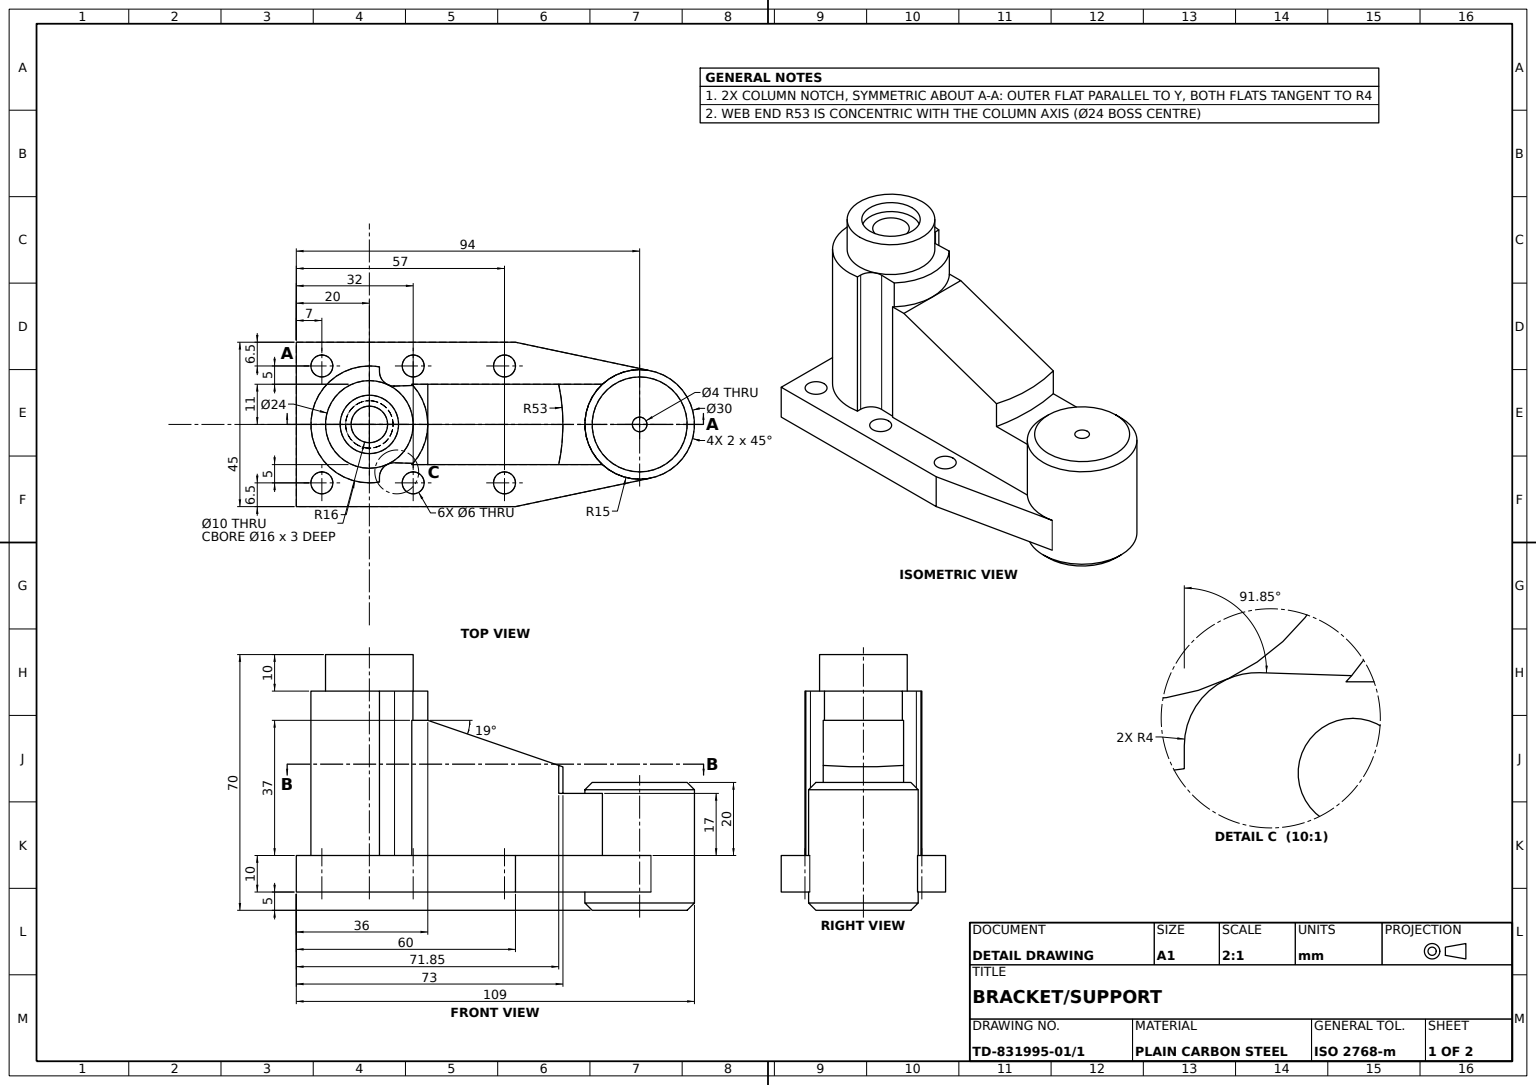
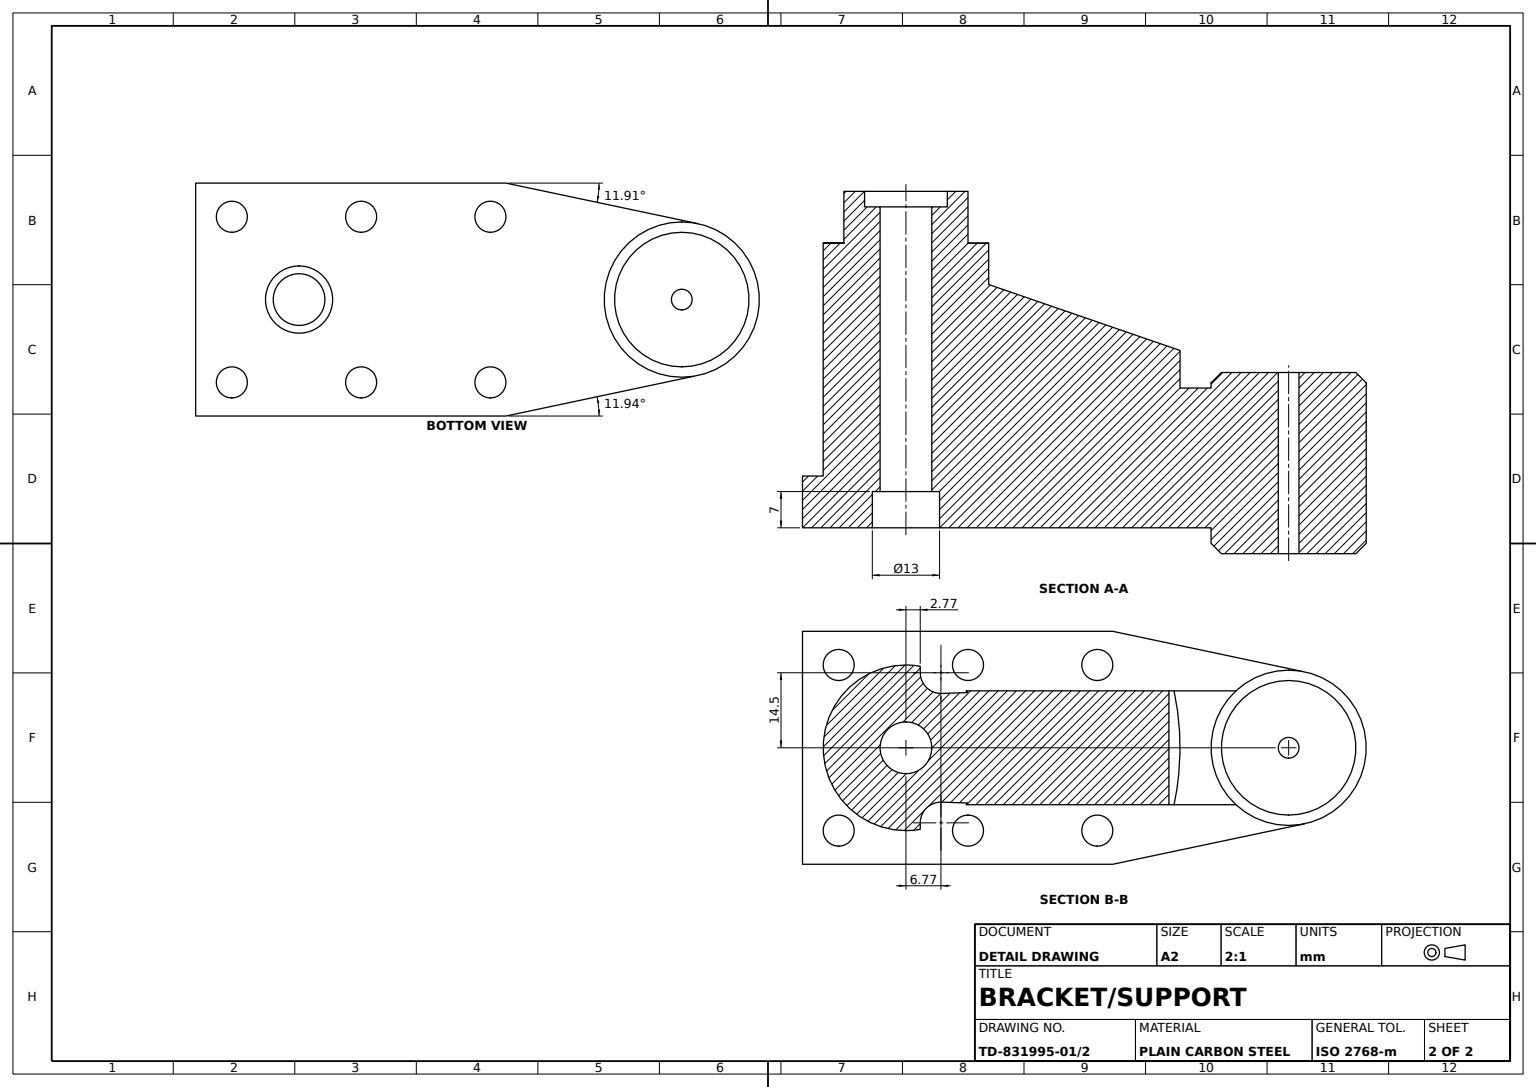
SolidWorks part; units mm, degrees
material "Plain Carbon Steel"
ref_plane "Front Plane" through (0, 0, 0) normal (0, 0, 1) x (1, 0, 0)
ref_plane "Top Plane" through (0, 0, 0) normal (0, 1, 0) x (1, 0, 0)
ref_plane "Right Plane" through (0, 0, 0) normal (1, 0, 0) x (0, 0, -1)
sketch "Pivot Hub Sketch" plane through (0, 0, 0) normal (0, 1, 0) x (1, 0, 0)
  circle A0 centre (0, 0) radius 15
  dimension "D1" = 30
extrude "Pivot Hub Ø30" add sketch "Pivot Hub Sketch" along normal blind 35
ref_plane "Plane1" through (0, 5, 0) normal (0, 1, 0) x (1, 0, 0)
sketch "Base Plate Sketch" plane through (0, 5, 0) normal (0, 1, 0) x (1, 0, 0)
  line L1 (-94, 0) -> (-94, 22.5)
  line L2 (-94, 22.5) -> (-34, 22.5)
  line L3 (-34, 22.5) -> (2.3279, 14.8183)
  line L4 (-94, 0) -> (-94, -22.5)
  line L5 (-94, -22.5) -> (-34, -22.5)
  line L6 (-34, -22.5) -> (3.0952, -14.6772)
  circle A0 centre (0, 0) radius 15 construction
  arc A1 (2.3279, 14.8183) -> (3.0952, -14.6772) centre (0, 0) ccw
  dimension "D1" = 45
  dimension "D2" = 60
  dimension "D3" = 36.3279
  dimension "D4" = 94
  dimension "D5" = 22.5
  dimension "D6" = 40.7707
  dimension "D7" = 94
  dimension "D8" = 37.0952
extrude "Base Plate" add sketch "Base Plate Sketch" along normal blind 10
sketch "Column Sketch" plane through (0, 15, 0) normal (0, 1, 0) x (1, 0, 0)
  circle A0 centre (-74, 0) radius 16
  dimension "D1" = 32
  dimension "D2" = 74
extrude "Column Ø32" add sketch "Column Sketch" along normal blind 45
sketch "Web Sketch" plane through (0, 15, 0) normal (0, 1, 0) x (1, 0, 0)
  line L0 (-74, 11) -> (-22.1541, 11)
  line L1 (-74, -11) -> (-22.1541, -11)
  arc A0 (-74, 11) -> (-74, -11) centre (-74, 0) ccw
  arc A1 (-22.1541, -11) -> (-22.1541, 11) centre (-74, 0) ccw
  dimension "D1" = 11
  dimension "D2" = 53
extrude "Sloped Web" add sketch "Web Sketch" along normal blind 37
sketch "Web Trim Sketch" plane through (0, 0, 11) normal (0, 0, 1) x (1, 0, 0)
  line L2 (-62.381, 52) -> (-62.381, 15) construction
  line L3 (-58, 52) -> (-22.1541, 52)
  line L7 (-58, 52) -> (-16.5018, 37.711)
  line L8 (-22.1541, 52) -> (-16.5018, 52)
  line L9 (-16.5018, 52) -> (-16.5018, 37.711)
  line L10 (-62.381, 52) -> (-22.1541, 52) construction
  dimension "D1" = 45.8793
  dimension "D2" = 14.289
extrude "Web Trim Cut" cut sketch "Web Trim Sketch" against normal blind 37
sketch "Web Pad Sketch" plane through (0, 15, 0) normal (0, 1, 0) x (1, 0, 0)
  line L0 (-22.1541, 11) -> (-1.8695, 11)
  line L1 (-1.8695, 11) -> (-1.8695, -11)
  line L2 (-1.8695, -11) -> (-22.1541, -11)
  arc A0 (-22.1541, 11) -> (-22.1541, -11) centre (-74, 0) cw
  dimension "D1" = 53
  dimension "D2" = 72.1305
extrude "Web Pad" add sketch "Web Pad Sketch" along normal blind 17
chamfer "Hub Chamfer A" distance 2 angle 45 1 edges at (0, 35, 15)
chamfer "Hub Chamfer B" distance 2 angle 45 1 edges at (0, 0, 15)
sketch "Hub Pin Hole Sketch" plane through (0, 35, 0) normal (0, 1, 0) x (1, 0, 0)
  circle A0 centre (0, 0) radius 2
  dimension "D1" = 4
extrude "Hub Pin Hole Ø4" cut sketch "Hub Pin Hole Sketch" against normal blind 39
sketch "Column Top Boss Sketch" plane through (0, 60, 0) normal (0, 1, 0) x (1, 0, 0)
  circle A0 centre (-74, 0) radius 12
  dimension "D1" = 24
extrude "Column Top Boss Ø24" add sketch "Column Top Boss Sketch" along normal blind 10
sketch "Top Counterbore Sketch" plane through (0, 70, 0) normal (0, 1, 0) x (1, 0, 0)
  circle A0 centre (-74, 0) radius 8
  dimension "D1" = 16
extrude "Top Counterbore Ø16" cut sketch "Top Counterbore Sketch" against normal blind 3
sketch "Column Bore Sketch" plane through (0, 67, 0) normal (0, 1, 0) x (1, 0, 0)
  circle A0 centre (-74, 0) radius 5
  dimension "D1" = 10
extrude "Column Bore Ø10" cut sketch "Column Bore Sketch" against normal blind 106
sketch "Bottom Counterbore Sketch" plane through (0, 5, 0) normal (0, -1, 0) x (1, 0, 0)
  circle A0 centre (-74, 0) radius 6.5
  dimension "D1" = 13
extrude "Bottom Counterbore Ø13" cut sketch "Bottom Counterbore Sketch" against normal blind 7
sketch "Column Slot Sketch" plane through (0, 60, 0) normal (0, 1, 0) x (1, 0, 0)
  line L0 (-67.105, -10.501) -> (-62.0712, -10.6632)
  line L2 (-69.2042, 11) -> (-69.1723, 11)
  line L5 (-71.2338, -15.7591) -> (-71.2338, -14.4989)
  line L6 (-71.2338, 15.7591) -> (-71.2338, 14.4989)
  line L7 (-67.105, 10.501) -> (-62.0712, 10.6632)
  arc A1 (-62.0712, 10.6632) -> (-71.2338, 15.7591) centre (-74, 0) ccw
  arc A2 (-71.2338, -14.4989) -> (-67.105, -10.501) centre (-67.2338, -14.4989) cw
  arc A3 (-68.9254, 10.8742) -> (-69.2042, 11) centre (-74, 0) ccw
  arc A4 (-71.2338, 14.4989) -> (-67.105, 10.501) centre (-67.2338, 14.4989) ccw
  arc A5 (-71.2338, -15.7591) -> (-62.0712, -10.6632) centre (-74, 0) ccw
  circle A6 centre (-74, 0) radius 12 construction
  circle M5 centre (-74, 0) radius 16
  dimension "D1" = 32
  dimension "D2" = 2.7662
  dimension "D3" = 4
  dimension "D4" = 24
  dimension "D5" = 4.7958
  dimension "D6" = 4.8277
  dimension "D7" = 6.895
  dimension "D8" = 10.501
extrude "Column Slot" cut sketch "Column Slot Sketch" against normal up to vertex contours L6 A4 L7 M5 | A2 L5 L0 M5
sketch "Base Mounting Holes Sketch" plane through (0, 15, 0) normal (0, 1, 0) x (1, 0, 0)
  circle A2 centre (-87, -16) radius 3
  circle A3 centre (-62, -16) radius 3
  circle A4 centre (-37, -16) radius 3
  circle A5 centre (-87, 16) radius 3
  circle A6 centre (-37, 16) radius 3
  circle A7 centre (-62, 16) radius 3
  circle A8 centre (-74, 0) radius 5 construction
  dimension "D1" = 6
  dimension "D2" = 6
  dimension "D3" = 6
  dimension "D10" = 6
  dimension "D11" = 6
  dimension "D12" = 6
  dimension "D13" = 32
  dimension "D4" = 87
  dimension "D5" = 16
  dimension "D6" = 62
  dimension "D7" = 16
  dimension "D8" = 37
  dimension "D9" = 16
  dimension "D14" = 40.3113
  dimension "D15" = 62
  dimension "D16" = 32
  dimension "D17" = 32
  dimension "D18" = 13
extrude "Base Mounting Holes Ø6" cut sketch "Base Mounting Holes Sketch" against normal blind 196
